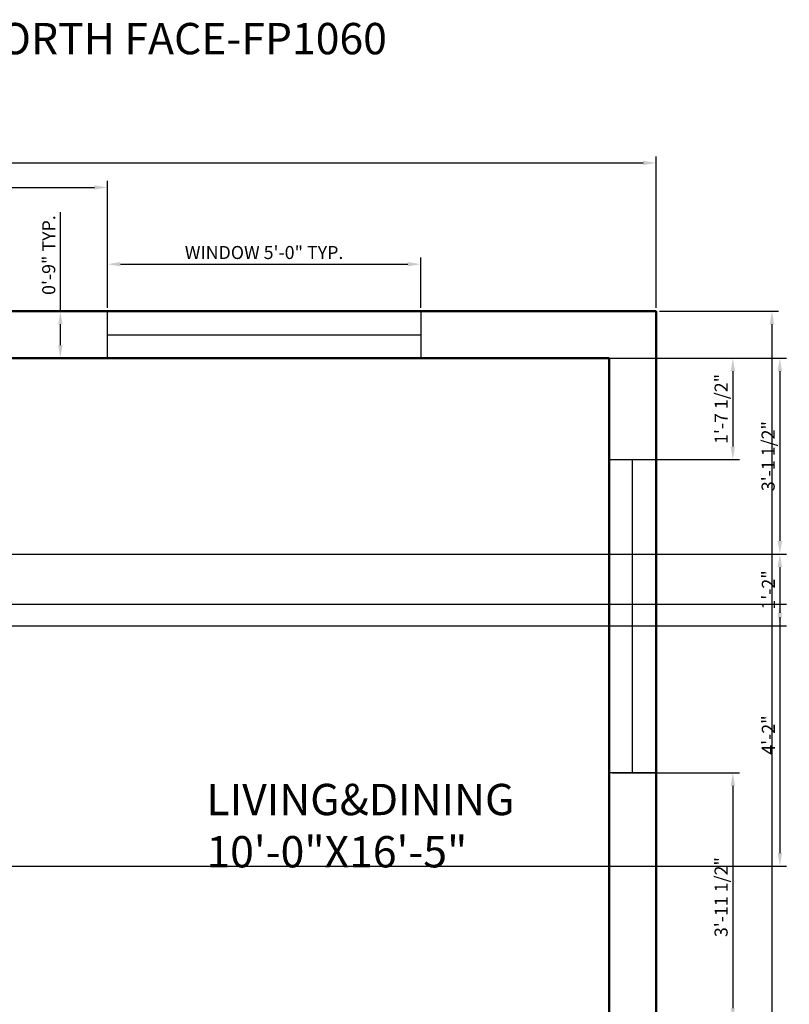
# Model space of a CAD drawing. Units: inches. Extents: x 3242 to 3618, y 1365 to 1814.
# Tile 6 of 6: x 3471 to 3618, y 1626 to 1814. Entities that reach past the tile are written whole.
import ezdxf

# ---------------------------------------------------------------- set-up
doc = ezdxf.new("R2010")
doc.units = ezdxf.units.IN
for name, color, linetype, lineweight in [('A-ANNO-DIMS', 2, 'Continuous', 18), ('A-ANNO-TEXT', 7, 'Continuous', 25), ('A-AREA-IDEN', 7, 'Continuous', 25), ('A-GLAZ', 5, 'Continuous', 25), ('A-WALL', 7, 'Continuous', 50)]:
    doc.layers.add(name, color=color, linetype=linetype, lineweight=lineweight)
doc.styles.get("Standard").update_dxf_attribs({"font": 'arial.ttf'})
doc.dimstyles.new('ISO-25', dxfattribs={"dimtxt": 2.5, "dimasz": 2.5, "dimexe": 1.25, "dimexo": 0.625, "dimtad": 1, "dimdec": 0, "dimlunit": 3, "dimtxsty": 'Standard', "dimcen": 2.5, "dimadec": 0, "dimazin": 0, "dimtfac": 1, "dimtdec": 0, "dimtmove": 0, "dimatfit": 3, "dimfxl": 1, "dimarcsym": 0})

# ---------------------------------------------------------------- blocks, each defined once
blk = doc.blocks.new('*D3')
at = {"layer": 'A-ANNO-DIMS', "color": 0, "lineweight": -2, "transparency": 16777216}
for p, q in [((3271.48, 1759.28), (3271.48, 1788.3)), ((3592.48, 1759.28), (3592.48, 1788.3)), ((3273.98, 1787.05), (3589.98, 1787.05))]:
    blk.add_line(p, q, dxfattribs=at)
at = {"layer": 'A-ANNO-DIMS', "color": 0, "transparency": 16777216}
for points in [[(3273.98, 1787.47), (3273.98, 1786.64), (3271.48, 1787.05)], [(3589.98, 1787.47), (3589.98, 1786.64), (3592.48, 1787.05)]]:
    blk.add_solid(points, dxfattribs=at)
at = {"layer": 'Defpoints', "color": 0, "transparency": 16777216}
for p in [(3592.48, 1787.05), (3271.48, 1758.66), (3592.48, 1758.66)]:
    blk.add_point(p, dxfattribs=at)
at = {"layer": 'A-ANNO-DIMS', "color": 0, "transparency": 16777216, "insert": (3431.98, 1790.74), "char_height": 6, "attachment_point": 5}
blk.add_mtext('26\'-9"', dxfattribs=at)
blk = doc.blocks.new('*D4')
at = {"layer": 'A-ANNO-DIMS', "color": 0, "lineweight": -2, "transparency": 16777216}
for p, q in [((3593.11, 1758.66), (3615.91, 1758.66)), ((3614.66, 1756.16), (3614.66, 1404.16)), ((3593.11, 1401.66), (3615.91, 1401.66))]:
    blk.add_line(p, q, dxfattribs=at)
at = {"layer": 'A-ANNO-DIMS', "color": 0, "transparency": 16777216}
for points in [[(3614.24, 1756.16), (3615.08, 1756.16), (3614.66, 1758.66)], [(3614.24, 1404.16), (3615.08, 1404.16), (3614.66, 1401.66)]]:
    blk.add_solid(points, dxfattribs=at)
at = {"layer": 'Defpoints', "color": 0, "transparency": 16777216}
for p in [(3592.48, 1758.66), (3592.48, 1401.66), (3614.66, 1401.66)]:
    blk.add_point(p, dxfattribs=at)
at = {"layer": 'A-ANNO-DIMS', "color": 0, "transparency": 16777216, "insert": (3610.97, 1580.16), "char_height": 6, "attachment_point": 5, "rotation": 90}
blk.add_mtext('29\'-9"', dxfattribs=at)
blk = doc.blocks.new('WINDOW-60IN')
for p, q in [((0, 9), (60, 9)), ((0, 0), (0, 9)), ((60, 9), (60, 0)), ((0, 4.5), (60, 4.5)), ((60, 0), (0, 0))]:
    blk.add_line(p, q)
blk = doc.blocks.new('*D13')
at = {"layer": 'A-ANNO-DIMS', "color": 0, "lineweight": -2, "transparency": 16777216}
for p, q in [((3487.43, 1759.28), (3487.43, 1768.91)), ((3547.43, 1759.28), (3547.43, 1768.91)), ((3489.93, 1767.66), (3544.93, 1767.66))]:
    blk.add_line(p, q, dxfattribs=at)
at = {"layer": 'A-ANNO-DIMS', "color": 0, "transparency": 16777216}
for points in [[(3489.93, 1768.07), (3489.93, 1767.24), (3487.43, 1767.66)], [(3544.93, 1768.07), (3544.93, 1767.24), (3547.43, 1767.66)]]:
    blk.add_solid(points, dxfattribs=at)
at = {"layer": 'Defpoints', "color": 0, "transparency": 16777216}
for p in [(3547.43, 1767.66), (3487.43, 1758.66), (3547.43, 1758.66)]:
    blk.add_point(p, dxfattribs=at)
at = {"layer": 'A-ANNO-DIMS', "color": 0, "transparency": 16777216, "insert": (3517.43, 1769.57), "char_height": 2.5, "attachment_point": 5}
blk.add_mtext('WINDOW 5\'-0" TYP.', dxfattribs=at)
blk = doc.blocks.new('*D14')
at = {"layer": 'A-ANNO-DIMS', "color": 0, "lineweight": -2, "transparency": 16777216}
for p, q in [((3478.43, 1758.66), (3478.43, 1777.64)), ((3486.8, 1758.66), (3477.18, 1758.66)), ((3478.43, 1752.16), (3478.43, 1756.16)), ((3486.8, 1749.66), (3477.18, 1749.66))]:
    blk.add_line(p, q, dxfattribs=at)
at = {"layer": 'A-ANNO-DIMS', "color": 0, "transparency": 16777216}
for points in [[(3478.01, 1756.16), (3478.84, 1756.16), (3478.43, 1758.66)], [(3478.01, 1752.16), (3478.84, 1752.16), (3478.43, 1749.66)]]:
    blk.add_solid(points, dxfattribs=at)
at = {"layer": 'Defpoints', "color": 0, "transparency": 16777216}
for p in [(3478.43, 1758.66), (3487.43, 1758.66), (3487.43, 1749.66)]:
    blk.add_point(p, dxfattribs=at)
at = {"layer": 'A-ANNO-DIMS', "color": 0, "transparency": 16777216, "insert": (3476.52, 1769.4), "char_height": 2.5, "attachment_point": 5, "rotation": 90}
blk.add_mtext('0\'-9" TYP.', dxfattribs=at)
blk = doc.blocks.new('*D34')
at = {"layer": 'A-ANNO-DIMS', "color": 0, "lineweight": -2, "transparency": 16777216}
for p, q in [((3419.36, 1759.28), (3419.36, 1783.61)), ((3421.86, 1782.36), (3484.93, 1782.36)), ((3487.43, 1759.28), (3487.43, 1783.61))]:
    blk.add_line(p, q, dxfattribs=at)
at = {"layer": 'A-ANNO-DIMS', "color": 0, "transparency": 16777216}
for points in [[(3421.86, 1782.77), (3421.86, 1781.94), (3419.36, 1782.36)], [(3484.93, 1782.77), (3484.93, 1781.94), (3487.43, 1782.36)]]:
    blk.add_solid(points, dxfattribs=at)
at = {"layer": 'Defpoints', "color": 0, "transparency": 16777216}
for p in [(3487.43, 1782.36), (3419.36, 1758.66), (3487.43, 1758.66)]:
    blk.add_point(p, dxfattribs=at)
at = {"layer": 'A-ANNO-DIMS', "color": 0, "transparency": 16777216, "insert": (3453.39, 1784.26), "char_height": 2.5, "attachment_point": 5}
blk.add_mtext('5\'-8"', dxfattribs=at)
blk = doc.blocks.new('*D35')
at = {"layer": 'A-ANNO-DIMS', "color": 0, "lineweight": -2, "transparency": 16777216}
for p, q in [((3584.11, 1749.66), (3608.43, 1749.66)), ((3607.18, 1747.16), (3607.18, 1732.73)), ((3584.11, 1730.23), (3608.43, 1730.23))]:
    blk.add_line(p, q, dxfattribs=at)
at = {"layer": 'A-ANNO-DIMS', "color": 0, "transparency": 16777216}
for points in [[(3606.76, 1747.16), (3607.6, 1747.16), (3607.18, 1749.66)], [(3606.76, 1732.73), (3607.6, 1732.73), (3607.18, 1730.23)]]:
    blk.add_solid(points, dxfattribs=at)
at = {"layer": 'Defpoints', "color": 0, "transparency": 16777216}
for p in [(3583.48, 1749.66), (3583.48, 1730.23), (3607.18, 1730.23)]:
    blk.add_point(p, dxfattribs=at)
at = {"layer": 'A-ANNO-DIMS', "color": 0, "transparency": 16777216, "insert": (3605.26, 1739.94), "char_height": 2.5, "attachment_point": 5, "rotation": 90}
blk.add_mtext('1\'-7 1/2"', dxfattribs=at)
blk = doc.blocks.new('*D36')
at = {"layer": 'A-ANNO-DIMS', "color": 0, "lineweight": -2, "transparency": 16777216}
for p, q in [((3584.11, 1670.23), (3608.43, 1670.23)), ((3607.18, 1667.73), (3607.18, 1625.17)), ((3584.11, 1622.67), (3608.43, 1622.67))]:
    blk.add_line(p, q, dxfattribs=at)
at = {"layer": 'A-ANNO-DIMS', "color": 0, "transparency": 16777216}
for points in [[(3606.76, 1667.73), (3607.6, 1667.73), (3607.18, 1670.23)], [(3606.76, 1625.17), (3607.6, 1625.17), (3607.18, 1622.67)]]:
    blk.add_solid(points, dxfattribs=at)
at = {"layer": 'Defpoints', "color": 0, "transparency": 16777216}
for p in [(3583.48, 1670.23), (3583.48, 1622.67), (3607.18, 1622.67)]:
    blk.add_point(p, dxfattribs=at)
at = {"layer": 'A-ANNO-DIMS', "color": 0, "transparency": 16777216, "insert": (3605.26, 1646.45), "char_height": 2.5, "attachment_point": 5, "rotation": 90}
blk.add_mtext('3\'-11 1/2"', dxfattribs=at)
blk = doc.blocks.new('*D49')
at = {"layer": 'A-ANNO-DIMS', "color": 0, "lineweight": -2, "transparency": 16777216}
for p, q in [((3395.11, 1702.58), (3617.43, 1702.58)), ((3616.18, 1700.08), (3616.18, 1654.87)), ((3395.11, 1652.37), (3617.43, 1652.37))]:
    blk.add_line(p, q, dxfattribs=at)
at = {"layer": 'A-ANNO-DIMS', "color": 0, "transparency": 16777216}
for points in [[(3615.76, 1700.08), (3616.6, 1700.08), (3616.18, 1702.58)], [(3615.76, 1654.87), (3616.6, 1654.87), (3616.18, 1652.37)]]:
    blk.add_solid(points, dxfattribs=at)
at = {"layer": 'Defpoints', "color": 0, "transparency": 16777216}
for p in [(3394.48, 1702.58), (3394.48, 1652.37), (3616.18, 1652.37)]:
    blk.add_point(p, dxfattribs=at)
at = {"layer": 'A-ANNO-DIMS', "color": 0, "transparency": 16777216, "insert": (3614.3, 1677.48), "char_height": 2.5, "attachment_point": 5, "rotation": 90}
blk.add_mtext('4\'-2"', dxfattribs=at)
blk = doc.blocks.new('*D50')
at = {"layer": 'A-ANNO-DIMS', "color": 0, "lineweight": -2, "transparency": 16777216}
for p, q in [((3348.02, 1712.15), (3617.43, 1712.15)), ((3616.18, 1709.65), (3616.18, 1700.88)), ((3348.02, 1698.38), (3617.43, 1698.38))]:
    blk.add_line(p, q, dxfattribs=at)
at = {"layer": 'A-ANNO-DIMS', "color": 0, "transparency": 16777216}
for points in [[(3615.76, 1709.65), (3616.6, 1709.65), (3616.18, 1712.15)], [(3615.76, 1700.88), (3616.6, 1700.88), (3616.18, 1698.38)]]:
    blk.add_solid(points, dxfattribs=at)
at = {"layer": 'Defpoints', "color": 0, "transparency": 16777216}
for p in [(3347.39, 1712.15), (3347.39, 1698.38), (3616.18, 1698.38)]:
    blk.add_point(p, dxfattribs=at)
at = {"layer": 'A-ANNO-DIMS', "color": 0, "transparency": 16777216, "insert": (3614.3, 1705.27), "char_height": 2.5, "attachment_point": 5, "rotation": 90}
blk.add_mtext('1\'-2"', dxfattribs=at)
blk = doc.blocks.new('*D58')
at = {"layer": 'A-ANNO-DIMS', "color": 0, "lineweight": -2, "transparency": 16777216}
for p, q in [((3333.61, 1749.66), (3617.43, 1749.66)), ((3616.18, 1747.16), (3616.18, 1714.65)), ((3336.54, 1712.15), (3617.43, 1712.15))]:
    blk.add_line(p, q, dxfattribs=at)
at = {"layer": 'A-ANNO-DIMS', "color": 0, "transparency": 16777216}
for points in [[(3615.76, 1747.16), (3616.6, 1747.16), (3616.18, 1749.66)], [(3615.76, 1714.65), (3616.6, 1714.65), (3616.18, 1712.15)]]:
    blk.add_solid(points, dxfattribs=at)
at = {"layer": 'Defpoints', "color": 0, "transparency": 16777216}
for p in [(3332.98, 1749.66), (3335.91, 1712.15), (3616.18, 1712.15)]:
    blk.add_point(p, dxfattribs=at)
at = {"layer": 'A-ANNO-DIMS', "color": 0, "transparency": 16777216, "insert": (3614.26, 1730.9), "char_height": 2.5, "attachment_point": 5, "rotation": 90}
blk.add_mtext('3\'-1 1/2"', dxfattribs=at)

msp = doc.modelspace()

# ---------------------------------------------------------------- linework, layer by layer
at = {"layer": 'A-WALL'}
for p, q in [((3271.48, 1758.66), (3592.48, 1758.66)), ((3592.48, 1758.66), (3592.48, 1401.66)), ((3280.48, 1749.66), (3583.48, 1749.66)), ((3583.48, 1749.66), (3583.48, 1557.66))]:
    msp.add_line(p, q, dxfattribs=at)

# ---------------------------------------------------------------- block references
at = {"layer": 'A-GLAZ'}
msp.add_blockref('WINDOW-60IN', (3487.43, 1749.65), dxfattribs=at)
at = {"layer": 'A-GLAZ', "rotation": 89.99999999999928}
msp.add_blockref('WINDOW-60IN', (3592.48, 1670.23), dxfattribs=at)

# ---------------------------------------------------------------- texts
at = {"layer": 'A-ANNO-TEXT', "insert": (3349.47, 1813.86), "char_height": 6, "attachment_point": 1}
msp.add_mtext('27X30[810sq ft]HOUSE PLAN-NORTH FACE-FP1060', dxfattribs=at)
at = {"layer": 'A-AREA-IDEN', "insert": (3506.39, 1668.14), "char_height": 6, "attachment_point": 1}
msp.add_mtext('LIVING&DINING\\P10\'-0"X16\'-5"', dxfattribs=at)

# ---------------------------------------------------------------- dimensions: what is measured, and where the dimension line sits
at = {"layer": 'A-ANNO-DIMS'}
for base, p1, p2, override, picture, middle in [((3592.48, 1787.05), (3271.48, 1758.66), (3592.48, 1758.66), {"dimtxt": 6, "dimclrd": 0, "dimclre": 0, "dimclrt": 0}, '*D3', (3431.98, 1790.74)), ((3487.43, 1782.36), (3419.36, 1758.66), (3487.43, 1758.66), {"dimdec": 1, "dimlfac": 1, "dimrnd": 0, "dimzin": 1, "dimdsep": 46, "dimlunit": 4, "dimfrac": 2}, '*D34', (3453.39, 1784.26))]:
    dim = msp.add_linear_dim(base=base, p1=p1, p2=p2, dimstyle='ISO-25', override=override, dxfattribs=at)
    dim.commit()
    dim.dimension.update_dxf_attribs({"geometry": picture, "text_midpoint": middle})
dim = msp.add_linear_dim(base=(3478.43, 1758.66), p1=(3487.43, 1749.66), p2=(3487.43, 1758.66), angle=90, text='<> TYP.', dimstyle='ISO-25', override={"dimdec": 1, "dimlfac": 1, "dimrnd": 0, "dimzin": 1, "dimdsep": 46, "dimlunit": 4, "dimfrac": 2}, dxfattribs=at)
dim.commit()
dim.dimension.update_dxf_attribs({"geometry": '*D14', "text_midpoint": (3476.52, 1769.4)})
dim = msp.add_linear_dim(base=(3547.43, 1767.66), p1=(3487.43, 1758.66), p2=(3547.43, 1758.66), text='WINDOW <> TYP.', dimstyle='ISO-25', override={"dimdec": 1, "dimlfac": 1, "dimrnd": 0, "dimzin": 1, "dimdsep": 46, "dimlunit": 4, "dimfrac": 2}, dxfattribs=at)
dim.commit()
dim.dimension.update_dxf_attribs({"geometry": '*D13', "text_midpoint": (3517.43, 1769.57)})
for base, p1, p2, angle, override, picture, middle in [((3614.66, 1401.66), (3592.48, 1758.66), (3592.48, 1401.66), 90, {"dimtxt": 6, "dimclrd": 0, "dimclre": 0, "dimclrt": 0}, '*D4', (3610.97, 1580.16)), ((3616.18, 1712.15), (3332.98, 1749.66), (3335.91, 1712.15), 90, {"dimdec": 1, "dimlfac": 1, "dimrnd": 0, "dimzin": 1, "dimdsep": 46, "dimlunit": 4, "dimfrac": 2}, '*D58', (3614.26, 1730.9)), ((3607.18, 1730.23), (3583.48, 1749.66), (3583.48, 1730.23), 270, {"dimdec": 1, "dimlfac": 1, "dimrnd": 0, "dimzin": 1, "dimdsep": 46, "dimlunit": 4, "dimfrac": 2}, '*D35', (3605.26, 1739.94)), ((3616.18, 1698.38), (3347.39, 1712.15), (3347.39, 1698.38), 90, {"dimdec": 1, "dimlfac": 1, "dimrnd": 0, "dimzin": 1, "dimdsep": 46, "dimlunit": 4, "dimfrac": 2}, '*D50', (3614.3, 1705.27)), ((3616.18, 1652.37), (3394.48, 1702.58), (3394.48, 1652.37), 90, {"dimdec": 1, "dimlfac": 1, "dimrnd": 0, "dimzin": 1, "dimdsep": 46, "dimlunit": 4, "dimfrac": 2}, '*D49', (3614.3, 1677.48)), ((3607.18, 1622.67), (3583.48, 1670.23), (3583.48, 1622.67), 270, {"dimdec": 1, "dimlfac": 1, "dimrnd": 0, "dimzin": 1, "dimdsep": 46, "dimlunit": 4, "dimfrac": 2}, '*D36', (3605.26, 1646.45))]:
    dim = msp.add_linear_dim(base=base, p1=p1, p2=p2, angle=angle, dimstyle='ISO-25', override=override, dxfattribs=at)
    dim.commit()
    dim.dimension.update_dxf_attribs({"geometry": picture, "text_midpoint": middle})

doc.saveas('drawing.dxf')
